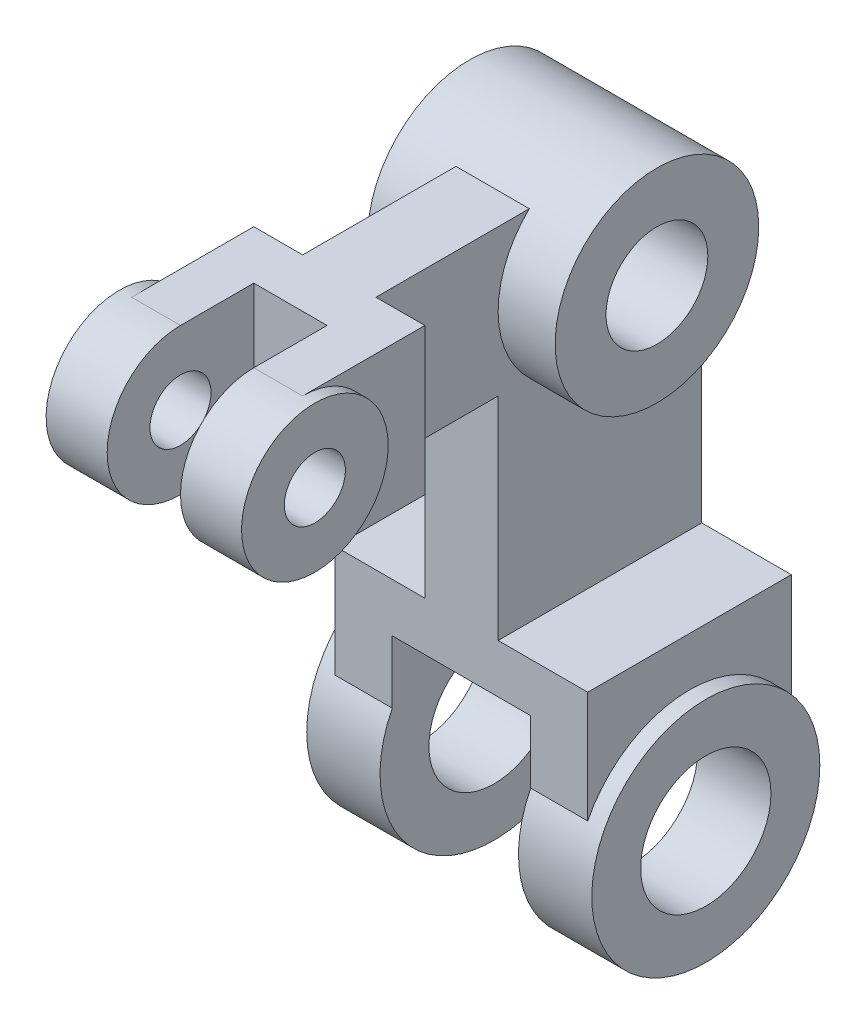
ISO-10303-21;
HEADER;
FILE_DESCRIPTION(('STEP AP214'),'2;1');
FILE_NAME('part.step','',(''),(''),'','','');
FILE_SCHEMA(('AUTOMOTIVE_DESIGN { 1 0 10303 214 1 1 1 1 }'));
ENDSEC;
DATA;
#1=APPLICATION_CONTEXT('core data for automotive mechanical design processes');
#2=APPLICATION_PROTOCOL_DEFINITION('international standard','automotive_design',2000,#1);
#3=PRODUCT_CONTEXT('',#1,'mechanical');
#4=PRODUCT('Part','Part','',(#3));
#5=PRODUCT_RELATED_PRODUCT_CATEGORY('part','',(#4));
#6=PRODUCT_DEFINITION_FORMATION('','',#4);
#7=PRODUCT_DEFINITION_CONTEXT('part definition',#1,'design');
#8=PRODUCT_DEFINITION('design','',#6,#7);
#9=PRODUCT_DEFINITION_SHAPE('','',#8);
#10=(LENGTH_UNIT() NAMED_UNIT(*) SI_UNIT(.MILLI.,.METRE.));
#11=(NAMED_UNIT(*) PLANE_ANGLE_UNIT() SI_UNIT($,.RADIAN.));
#12=(NAMED_UNIT(*) SI_UNIT($,.STERADIAN.) SOLID_ANGLE_UNIT());
#13=UNCERTAINTY_MEASURE_WITH_UNIT(LENGTH_MEASURE(1.E-05),#10,'distance_accuracy_value','');
#14=(GEOMETRIC_REPRESENTATION_CONTEXT(3) GLOBAL_UNCERTAINTY_ASSIGNED_CONTEXT((#13)) GLOBAL_UNIT_ASSIGNED_CONTEXT((#10,
#11,#12)) REPRESENTATION_CONTEXT('',''));
#15=CARTESIAN_POINT('',(0.,0.,0.));
#16=DIRECTION('',(0.,0.,1.));
#17=DIRECTION('',(1.,0.,0.));
#18=AXIS2_PLACEMENT_3D('',#15,#16,#17);
#19=CARTESIAN_POINT('',(0.,0.,25.));
#20=DIRECTION('',(0.,0.,-1.));
#21=DIRECTION('',(-1.,0.,0.));
#22=AXIS2_PLACEMENT_3D('',#19,#20,#21);
#23=PLANE('',#22);
#24=DIRECTION('',(1.,0.,0.));
#25=VECTOR('',#24,1.);
#26=CARTESIAN_POINT('',(0.,92.,25.));
#27=LINE('',#26,#25);
#28=CARTESIAN_POINT('',(-9.,92.,25.));
#29=VERTEX_POINT('',#28);
#30=CARTESIAN_POINT('',(9.,92.,25.));
#31=VERTEX_POINT('',#30);
#32=EDGE_CURVE('E297',#29,#31,#27,.T.);
#33=ORIENTED_EDGE('',*,*,#32,.F.);
#34=DIRECTION('',(0.,-1.,0.));
#35=VECTOR('',#34,1.);
#36=CARTESIAN_POINT('',(-9.,110.,25.));
#37=LINE('',#36,#35);
#38=CARTESIAN_POINT('',(-8.99999999999999,40.,25.));
#39=VERTEX_POINT('',#38);
#40=EDGE_CURVE('E335',#29,#39,#37,.T.);
#41=ORIENTED_EDGE('',*,*,#40,.T.);
#42=DIRECTION('',(-1.,0.,0.));
#43=VECTOR('',#42,1.);
#44=CARTESIAN_POINT('',(-8.99999999999999,40.,25.));
#45=LINE('',#44,#43);
#46=CARTESIAN_POINT('',(-31.,40.,25.));
#47=VERTEX_POINT('',#46);
#48=EDGE_CURVE('E331',#39,#47,#45,.T.);
#49=ORIENTED_EDGE('',*,*,#48,.T.);
#50=DIRECTION('',(0.,-1.,0.));
#51=VECTOR('',#50,1.);
#52=CARTESIAN_POINT('',(-31.,40.,25.));
#53=LINE('',#52,#51);
#54=CARTESIAN_POINT('',(-31.,12.6095202129185,25.));
#55=VERTEX_POINT('',#54);
#56=EDGE_CURVE('E339',#47,#55,#53,.T.);
#57=ORIENTED_EDGE('',*,*,#56,.T.);
#58=DIRECTION('',(1.,0.,0.));
#59=VECTOR('',#58,1.);
#60=CARTESIAN_POINT('',(-35.,12.6095202129185,25.));
#61=LINE('',#60,#59);
#62=CARTESIAN_POINT('',(-17.,12.6095202129185,25.));
#63=VERTEX_POINT('',#62);
#64=EDGE_CURVE('E314',#55,#63,#61,.T.);
#65=ORIENTED_EDGE('',*,*,#64,.T.);
#66=DIRECTION('',(0.,1.,0.));
#67=VECTOR('',#66,1.);
#68=CARTESIAN_POINT('',(-17.,0.,25.));
#69=LINE('',#68,#67);
#70=CARTESIAN_POINT('',(-17.,28.,25.));
#71=VERTEX_POINT('',#70);
#72=EDGE_CURVE('E336',#63,#71,#69,.T.);
#73=ORIENTED_EDGE('',*,*,#72,.T.);
#74=DIRECTION('',(1.,0.,0.));
#75=VECTOR('',#74,1.);
#76=CARTESIAN_POINT('',(-17.,28.,25.));
#77=LINE('',#76,#75);
#78=CARTESIAN_POINT('',(17.,28.,25.));
#79=VERTEX_POINT('',#78);
#80=EDGE_CURVE('E343',#71,#79,#77,.T.);
#81=ORIENTED_EDGE('',*,*,#80,.T.);
#82=DIRECTION('',(0.,-1.,0.));
#83=VECTOR('',#82,1.);
#84=CARTESIAN_POINT('',(17.,0.,25.));
#85=LINE('',#84,#83);
#86=CARTESIAN_POINT('',(17.,12.6095202129185,25.));
#87=VERTEX_POINT('',#86);
#88=EDGE_CURVE('E341',#79,#87,#85,.T.);
#89=ORIENTED_EDGE('',*,*,#88,.T.);
#90=DIRECTION('',(-1.,0.,0.));
#91=VECTOR('',#90,1.);
#92=CARTESIAN_POINT('',(35.,12.6095202129185,25.));
#93=LINE('',#92,#91);
#94=CARTESIAN_POINT('',(31.,12.6095202129185,25.));
#95=VERTEX_POINT('',#94);
#96=EDGE_CURVE('E328',#95,#87,#93,.T.);
#97=ORIENTED_EDGE('',*,*,#96,.F.);
#98=DIRECTION('',(0.,1.,0.));
#99=VECTOR('',#98,1.);
#100=CARTESIAN_POINT('',(31.,40.,25.));
#101=LINE('',#100,#99);
#102=CARTESIAN_POINT('',(31.,40.,25.));
#103=VERTEX_POINT('',#102);
#104=EDGE_CURVE('E347',#95,#103,#101,.T.);
#105=ORIENTED_EDGE('',*,*,#104,.T.);
#106=DIRECTION('',(-1.,0.,0.));
#107=VECTOR('',#106,1.);
#108=CARTESIAN_POINT('',(8.99999999999999,40.,25.));
#109=LINE('',#108,#107);
#110=CARTESIAN_POINT('',(8.99999999999999,40.,25.));
#111=VERTEX_POINT('',#110);
#112=EDGE_CURVE('E346',#103,#111,#109,.T.);
#113=ORIENTED_EDGE('',*,*,#112,.T.);
#114=DIRECTION('',(0.,1.,0.));
#115=VECTOR('',#114,1.);
#116=CARTESIAN_POINT('',(9.,110.,25.));
#117=LINE('',#116,#115);
#118=EDGE_CURVE('E348',#111,#31,#117,.T.);
#119=ORIENTED_EDGE('',*,*,#118,.T.);
#120=EDGE_LOOP('',(#33,#41,#49,#57,#65,#73,#81,#89,#97,#105,#113,#119));
#121=FACE_BOUND('',#120,.T.);
#122=ADVANCED_FACE('F60',(#121),#23,.F.);
#123=CARTESIAN_POINT('',(23.,110.,0.));
#124=DIRECTION('',(-1.,0.,0.));
#125=DIRECTION('',(0.,0.,1.));
#126=AXIS2_PLACEMENT_3D('',#123,#124,#125);
#127=CYLINDRICAL_SURFACE('',#126,25.);
#128=CARTESIAN_POINT('',(23.,110.,0.));
#129=DIRECTION('',(1.,0.,0.));
#130=DIRECTION('',(0.,0.,-1.));
#131=AXIS2_PLACEMENT_3D('',#128,#129,#130);
#132=CIRCLE('',#131,25.);
#133=CARTESIAN_POINT('',(23.,110.,-25.));
#134=VERTEX_POINT('',#133);
#135=EDGE_CURVE('E402',#134,#134,#132,.T.);
#136=ORIENTED_EDGE('',*,*,#135,.F.);
#137=EDGE_LOOP('',(#136));
#138=FACE_BOUND('',#137,.T.);
#139=CARTESIAN_POINT('',(-23.,110.,0.));
#140=DIRECTION('',(1.,0.,0.));
#141=DIRECTION('',(0.,0.,-1.));
#142=AXIS2_PLACEMENT_3D('',#139,#140,#141);
#143=CIRCLE('',#142,25.);
#144=CARTESIAN_POINT('',(-23.,110.,-25.));
#145=VERTEX_POINT('',#144);
#146=EDGE_CURVE('E396',#145,#145,#143,.T.);
#147=ORIENTED_EDGE('',*,*,#146,.T.);
#148=EDGE_LOOP('',(#147));
#149=FACE_BOUND('',#148,.T.);
#150=DIRECTION('',(-1.,0.,0.));
#151=VECTOR('',#150,1.);
#152=CARTESIAN_POINT('',(23.,128.,17.3493515728975));
#153=LINE('',#152,#151);
#154=CARTESIAN_POINT('',(-9.,128.,17.3493515728975));
#155=VERTEX_POINT('',#154);
#156=CARTESIAN_POINT('',(9.,128.,17.3493515728975));
#157=VERTEX_POINT('',#156);
#158=EDGE_CURVE('E63',#155,#157,#153,.F.);
#159=ORIENTED_EDGE('',*,*,#158,.T.);
#160=CARTESIAN_POINT('',(9.,110.,0.));
#161=DIRECTION('',(-1.,0.,0.));
#162=DIRECTION('',(0.,-1.,0.));
#163=AXIS2_PLACEMENT_3D('',#160,#161,#162);
#164=CIRCLE('',#163,25.);
#165=CARTESIAN_POINT('',(9.,110.,-25.));
#166=VERTEX_POINT('',#165);
#167=EDGE_CURVE('E75',#166,#157,#164,.T.);
#168=ORIENTED_EDGE('',*,*,#167,.F.);
#169=DIRECTION('',(-1.,0.,0.));
#170=VECTOR('',#169,1.);
#171=CARTESIAN_POINT('',(-9.,110.,-25.));
#172=LINE('',#171,#170);
#173=CARTESIAN_POINT('',(-9.,110.,-25.));
#174=VERTEX_POINT('',#173);
#175=EDGE_CURVE('E332',#166,#174,#172,.T.);
#176=ORIENTED_EDGE('',*,*,#175,.T.);
#177=CARTESIAN_POINT('',(-9.,110.,0.));
#178=DIRECTION('',(1.,0.,0.));
#179=DIRECTION('',(0.,1.,0.));
#180=AXIS2_PLACEMENT_3D('',#177,#178,#179);
#181=CIRCLE('',#180,25.);
#182=EDGE_CURVE('E394',#155,#174,#181,.T.);
#183=ORIENTED_EDGE('',*,*,#182,.F.);
#184=EDGE_LOOP('',(#159,#168,#176,#183));
#185=FACE_BOUND('',#184,.T.);
#186=ADVANCED_FACE('F56',(#138,#149,#185),#127,.T.);
#187=CARTESIAN_POINT('',(23.,110.,0.));
#188=DIRECTION('',(-1.,0.,0.));
#189=DIRECTION('',(0.,0.,1.));
#190=AXIS2_PLACEMENT_3D('',#187,#188,#189);
#191=CYLINDRICAL_SURFACE('',#190,12.5);
#192=CARTESIAN_POINT('',(23.,110.,0.));
#193=DIRECTION('',(1.,0.,0.));
#194=DIRECTION('',(0.,0.,-1.));
#195=AXIS2_PLACEMENT_3D('',#192,#193,#194);
#196=CIRCLE('',#195,12.5);
#197=CARTESIAN_POINT('',(23.,110.,-12.5));
#198=VERTEX_POINT('',#197);
#199=EDGE_CURVE('E393',#198,#198,#196,.T.);
#200=ORIENTED_EDGE('',*,*,#199,.T.);
#201=EDGE_LOOP('',(#200));
#202=FACE_BOUND('',#201,.T.);
#203=CARTESIAN_POINT('',(-23.,110.,0.));
#204=DIRECTION('',(1.,0.,0.));
#205=DIRECTION('',(0.,0.,-1.));
#206=AXIS2_PLACEMENT_3D('',#203,#204,#205);
#207=CIRCLE('',#206,12.5);
#208=CARTESIAN_POINT('',(-23.,110.,-12.5));
#209=VERTEX_POINT('',#208);
#210=EDGE_CURVE('E391',#209,#209,#207,.T.);
#211=ORIENTED_EDGE('',*,*,#210,.F.);
#212=EDGE_LOOP('',(#211));
#213=FACE_BOUND('',#212,.T.);
#214=ADVANCED_FACE('F480',(#202,#213),#191,.F.);
#215=CARTESIAN_POINT('',(0.,0.,-25.));
#216=DIRECTION('',(0.,0.,-1.));
#217=DIRECTION('',(-1.,0.,0.));
#218=AXIS2_PLACEMENT_3D('',#215,#216,#217);
#219=PLANE('',#218);
#220=DIRECTION('',(1.,0.,0.));
#221=VECTOR('',#220,1.);
#222=CARTESIAN_POINT('',(-35.,12.6095202129185,-25.));
#223=LINE('',#222,#221);
#224=CARTESIAN_POINT('',(-31.,12.6095202129185,-25.));
#225=VERTEX_POINT('',#224);
#226=CARTESIAN_POINT('',(-17.,12.6095202129185,-25.));
#227=VERTEX_POINT('',#226);
#228=EDGE_CURVE('E313',#225,#227,#223,.T.);
#229=ORIENTED_EDGE('',*,*,#228,.F.);
#230=DIRECTION('',(0.,-1.,0.));
#231=VECTOR('',#230,1.);
#232=CARTESIAN_POINT('',(-31.,40.,-25.));
#233=LINE('',#232,#231);
#234=CARTESIAN_POINT('',(-31.,40.,-25.));
#235=VERTEX_POINT('',#234);
#236=EDGE_CURVE('E359',#235,#225,#233,.T.);
#237=ORIENTED_EDGE('',*,*,#236,.F.);
#238=DIRECTION('',(-1.,0.,0.));
#239=VECTOR('',#238,1.);
#240=CARTESIAN_POINT('',(-8.99999999999999,40.,-25.));
#241=LINE('',#240,#239);
#242=CARTESIAN_POINT('',(-8.99999999999999,40.,-25.));
#243=VERTEX_POINT('',#242);
#244=EDGE_CURVE('E356',#243,#235,#241,.T.);
#245=ORIENTED_EDGE('',*,*,#244,.F.);
#246=DIRECTION('',(0.,-1.,0.));
#247=VECTOR('',#246,1.);
#248=CARTESIAN_POINT('',(-9.,110.,-25.));
#249=LINE('',#248,#247);
#250=EDGE_CURVE('E358',#174,#243,#249,.T.);
#251=ORIENTED_EDGE('',*,*,#250,.F.);
#252=ORIENTED_EDGE('',*,*,#175,.F.);
#253=DIRECTION('',(0.,1.,0.));
#254=VECTOR('',#253,1.);
#255=CARTESIAN_POINT('',(9.,110.,-25.));
#256=LINE('',#255,#254);
#257=CARTESIAN_POINT('',(8.99999999999999,40.,-25.));
#258=VERTEX_POINT('',#257);
#259=EDGE_CURVE('E333',#258,#166,#256,.T.);
#260=ORIENTED_EDGE('',*,*,#259,.F.);
#261=DIRECTION('',(-1.,0.,0.));
#262=VECTOR('',#261,1.);
#263=CARTESIAN_POINT('',(8.99999999999999,40.,-25.));
#264=LINE('',#263,#262);
#265=CARTESIAN_POINT('',(31.,40.,-25.));
#266=VERTEX_POINT('',#265);
#267=EDGE_CURVE('E373',#266,#258,#264,.T.);
#268=ORIENTED_EDGE('',*,*,#267,.F.);
#269=DIRECTION('',(0.,1.,0.));
#270=VECTOR('',#269,1.);
#271=CARTESIAN_POINT('',(31.,40.,-25.));
#272=LINE('',#271,#270);
#273=CARTESIAN_POINT('',(31.,12.6095202129185,-25.));
#274=VERTEX_POINT('',#273);
#275=EDGE_CURVE('E371',#274,#266,#272,.T.);
#276=ORIENTED_EDGE('',*,*,#275,.F.);
#277=DIRECTION('',(-1.,0.,0.));
#278=VECTOR('',#277,1.);
#279=CARTESIAN_POINT('',(35.,12.6095202129185,-25.));
#280=LINE('',#279,#278);
#281=CARTESIAN_POINT('',(17.,12.6095202129185,-25.));
#282=VERTEX_POINT('',#281);
#283=EDGE_CURVE('E404',#274,#282,#280,.T.);
#284=ORIENTED_EDGE('',*,*,#283,.T.);
#285=DIRECTION('',(0.,-1.,0.));
#286=VECTOR('',#285,1.);
#287=CARTESIAN_POINT('',(17.,0.,-25.));
#288=LINE('',#287,#286);
#289=CARTESIAN_POINT('',(17.,28.,-25.));
#290=VERTEX_POINT('',#289);
#291=EDGE_CURVE('E366',#290,#282,#288,.T.);
#292=ORIENTED_EDGE('',*,*,#291,.F.);
#293=DIRECTION('',(1.,0.,0.));
#294=VECTOR('',#293,1.);
#295=CARTESIAN_POINT('',(-17.,28.,-25.));
#296=LINE('',#295,#294);
#297=CARTESIAN_POINT('',(-17.,28.,-25.));
#298=VERTEX_POINT('',#297);
#299=EDGE_CURVE('E364',#298,#290,#296,.T.);
#300=ORIENTED_EDGE('',*,*,#299,.F.);
#301=DIRECTION('',(0.,1.,0.));
#302=VECTOR('',#301,1.);
#303=CARTESIAN_POINT('',(-17.,0.,-25.));
#304=LINE('',#303,#302);
#305=EDGE_CURVE('E362',#227,#298,#304,.T.);
#306=ORIENTED_EDGE('',*,*,#305,.F.);
#307=EDGE_LOOP('',(#229,#237,#245,#251,#252,#260,#268,#276,#284,#292,#300,#306));
#308=FACE_BOUND('',#307,.T.);
#309=ADVANCED_FACE('F485',(#308),#219,.T.);
#310=CARTESIAN_POINT('',(23.,110.,0.));
#311=DIRECTION('',(1.,0.,0.));
#312=DIRECTION('',(0.,0.,-1.));
#313=AXIS2_PLACEMENT_3D('',#310,#311,#312);
#314=PLANE('',#313);
#315=ORIENTED_EDGE('',*,*,#135,.T.);
#316=EDGE_LOOP('',(#315));
#317=FACE_BOUND('',#316,.T.);
#318=ORIENTED_EDGE('',*,*,#199,.F.);
#319=EDGE_LOOP('',(#318));
#320=FACE_BOUND('',#319,.T.);
#321=ADVANCED_FACE('F482',(#317,#320),#314,.T.);
#322=CARTESIAN_POINT('',(-23.,110.,0.));
#323=DIRECTION('',(1.,0.,0.));
#324=DIRECTION('',(0.,0.,-1.));
#325=AXIS2_PLACEMENT_3D('',#322,#323,#324);
#326=PLANE('',#325);
#327=ORIENTED_EDGE('',*,*,#146,.F.);
#328=EDGE_LOOP('',(#327));
#329=FACE_BOUND('',#328,.T.);
#330=ORIENTED_EDGE('',*,*,#210,.T.);
#331=EDGE_LOOP('',(#330));
#332=FACE_BOUND('',#331,.T.);
#333=ADVANCED_FACE('F491',(#329,#332),#326,.F.);
#334=CARTESIAN_POINT('',(-9.,110.,25.));
#335=DIRECTION('',(1.,0.,0.));
#336=DIRECTION('',(0.,1.,0.));
#337=AXIS2_PLACEMENT_3D('',#334,#335,#336);
#338=PLANE('',#337);
#339=ORIENTED_EDGE('',*,*,#182,.T.);
#340=ORIENTED_EDGE('',*,*,#250,.T.);
#341=DIRECTION('',(0.,0.,-1.));
#342=VECTOR('',#341,1.);
#343=CARTESIAN_POINT('',(-8.99999999999999,40.,25.));
#344=LINE('',#343,#342);
#345=EDGE_CURVE('E389',#39,#243,#344,.T.);
#346=ORIENTED_EDGE('',*,*,#345,.F.);
#347=ORIENTED_EDGE('',*,*,#40,.F.);
#348=DIRECTION('',(0.,0.,1.));
#349=VECTOR('',#348,1.);
#350=CARTESIAN_POINT('',(-9.,92.,0.));
#351=LINE('',#350,#349);
#352=CARTESIAN_POINT('',(-8.99999999999999,92.,55.));
#353=VERTEX_POINT('',#352);
#354=EDGE_CURVE('E277',#29,#353,#351,.T.);
#355=ORIENTED_EDGE('',*,*,#354,.T.);
#356=DIRECTION('',(0.,-1.,0.));
#357=VECTOR('',#356,1.);
#358=CARTESIAN_POINT('',(-8.99999999999999,128.,55.));
#359=LINE('',#358,#357);
#360=CARTESIAN_POINT('',(-8.99999999999999,128.,55.));
#361=VERTEX_POINT('',#360);
#362=EDGE_CURVE('E285',#361,#353,#359,.T.);
#363=ORIENTED_EDGE('',*,*,#362,.F.);
#364=DIRECTION('',(0.,0.,1.));
#365=VECTOR('',#364,1.);
#366=CARTESIAN_POINT('',(-9.,128.,0.));
#367=LINE('',#366,#365);
#368=EDGE_CURVE('E247',#155,#361,#367,.T.);
#369=ORIENTED_EDGE('',*,*,#368,.F.);
#370=EDGE_LOOP('',(#339,#340,#346,#347,#355,#363,#369));
#371=FACE_BOUND('',#370,.T.);
#372=ADVANCED_FACE('F411',(#371),#338,.F.);
#373=CARTESIAN_POINT('',(-8.99999999999999,40.,25.));
#374=DIRECTION('',(0.,-1.,0.));
#375=DIRECTION('',(1.,0.,0.));
#376=AXIS2_PLACEMENT_3D('',#373,#374,#375);
#377=PLANE('',#376);
#378=ORIENTED_EDGE('',*,*,#244,.T.);
#379=DIRECTION('',(0.,0.,-1.));
#380=VECTOR('',#379,1.);
#381=CARTESIAN_POINT('',(-31.,40.,25.));
#382=LINE('',#381,#380);
#383=EDGE_CURVE('E384',#47,#235,#382,.T.);
#384=ORIENTED_EDGE('',*,*,#383,.F.);
#385=ORIENTED_EDGE('',*,*,#48,.F.);
#386=ORIENTED_EDGE('',*,*,#345,.T.);
#387=EDGE_LOOP('',(#378,#384,#385,#386));
#388=FACE_BOUND('',#387,.T.);
#389=ADVANCED_FACE('F636',(#388),#377,.F.);
#390=CARTESIAN_POINT('',(-31.,40.,25.));
#391=DIRECTION('',(1.,0.,0.));
#392=DIRECTION('',(0.,1.,0.));
#393=AXIS2_PLACEMENT_3D('',#390,#391,#392);
#394=PLANE('',#393);
#395=ORIENTED_EDGE('',*,*,#236,.T.);
#396=CARTESIAN_POINT('',(-31.,0.,0.));
#397=DIRECTION('',(1.,0.,0.));
#398=DIRECTION('',(0.,1.,0.));
#399=AXIS2_PLACEMENT_3D('',#396,#397,#398);
#400=CIRCLE('',#399,28.);
#401=EDGE_CURVE('E78',#225,#55,#400,.T.);
#402=ORIENTED_EDGE('',*,*,#401,.T.);
#403=ORIENTED_EDGE('',*,*,#56,.F.);
#404=ORIENTED_EDGE('',*,*,#383,.T.);
#405=EDGE_LOOP('',(#395,#402,#403,#404));
#406=FACE_BOUND('',#405,.T.);
#407=ADVANCED_FACE('F504',(#406),#394,.F.);
#408=CARTESIAN_POINT('',(-17.,0.,25.));
#409=DIRECTION('',(-1.,0.,0.));
#410=DIRECTION('',(0.,0.,1.));
#411=AXIS2_PLACEMENT_3D('',#408,#409,#410);
#412=PLANE('',#411);
#413=CARTESIAN_POINT('',(-17.,0.,0.));
#414=DIRECTION('',(1.,0.,0.));
#415=DIRECTION('',(0.,0.,-1.));
#416=AXIS2_PLACEMENT_3D('',#413,#414,#415);
#417=CIRCLE('',#416,16.);
#418=CARTESIAN_POINT('',(-17.,0.,-16.));
#419=VERTEX_POINT('',#418);
#420=EDGE_CURVE('E300',#419,#419,#417,.T.);
#421=ORIENTED_EDGE('',*,*,#420,.F.);
#422=EDGE_LOOP('',(#421));
#423=FACE_BOUND('',#422,.T.);
#424=ORIENTED_EDGE('',*,*,#72,.F.);
#425=CARTESIAN_POINT('',(-17.,0.,0.));
#426=DIRECTION('',(1.,0.,0.));
#427=DIRECTION('',(0.,0.,-1.));
#428=AXIS2_PLACEMENT_3D('',#425,#426,#427);
#429=CIRCLE('',#428,28.);
#430=EDGE_CURVE('E305',#63,#227,#429,.T.);
#431=ORIENTED_EDGE('',*,*,#430,.T.);
#432=ORIENTED_EDGE('',*,*,#305,.T.);
#433=DIRECTION('',(0.,0.,-1.));
#434=VECTOR('',#433,1.);
#435=CARTESIAN_POINT('',(-17.,28.,25.));
#436=LINE('',#435,#434);
#437=EDGE_CURVE('E382',#71,#298,#436,.T.);
#438=ORIENTED_EDGE('',*,*,#437,.F.);
#439=EDGE_LOOP('',(#424,#431,#432,#438));
#440=FACE_BOUND('',#439,.T.);
#441=ADVANCED_FACE('F507',(#423,#440),#412,.F.);
#442=CARTESIAN_POINT('',(-17.,28.,25.));
#443=DIRECTION('',(0.,1.,0.));
#444=DIRECTION('',(0.,0.,1.));
#445=AXIS2_PLACEMENT_3D('',#442,#443,#444);
#446=PLANE('',#445);
#447=ORIENTED_EDGE('',*,*,#299,.T.);
#448=DIRECTION('',(0.,0.,-1.));
#449=VECTOR('',#448,1.);
#450=CARTESIAN_POINT('',(17.,28.,25.));
#451=LINE('',#450,#449);
#452=EDGE_CURVE('E381',#79,#290,#451,.T.);
#453=ORIENTED_EDGE('',*,*,#452,.F.);
#454=ORIENTED_EDGE('',*,*,#80,.F.);
#455=ORIENTED_EDGE('',*,*,#437,.T.);
#456=EDGE_LOOP('',(#447,#453,#454,#455));
#457=FACE_BOUND('',#456,.T.);
#458=ADVANCED_FACE('F511',(#457),#446,.F.);
#459=CARTESIAN_POINT('',(17.,0.,25.));
#460=DIRECTION('',(1.,0.,0.));
#461=DIRECTION('',(0.,0.,-1.));
#462=AXIS2_PLACEMENT_3D('',#459,#460,#461);
#463=PLANE('',#462);
#464=CARTESIAN_POINT('',(17.,0.,0.));
#465=DIRECTION('',(1.,0.,0.));
#466=DIRECTION('',(0.,0.,-1.));
#467=AXIS2_PLACEMENT_3D('',#464,#465,#466);
#468=CIRCLE('',#467,16.);
#469=CARTESIAN_POINT('',(17.,0.,-16.));
#470=VERTEX_POINT('',#469);
#471=EDGE_CURVE('E316',#470,#470,#468,.T.);
#472=ORIENTED_EDGE('',*,*,#471,.T.);
#473=EDGE_LOOP('',(#472));
#474=FACE_BOUND('',#473,.T.);
#475=ORIENTED_EDGE('',*,*,#452,.T.);
#476=ORIENTED_EDGE('',*,*,#291,.T.);
#477=CARTESIAN_POINT('',(17.,0.,0.));
#478=DIRECTION('',(1.,0.,0.));
#479=DIRECTION('',(0.,0.,-1.));
#480=AXIS2_PLACEMENT_3D('',#477,#478,#479);
#481=CIRCLE('',#480,28.);
#482=EDGE_CURVE('E319',#87,#282,#481,.T.);
#483=ORIENTED_EDGE('',*,*,#482,.F.);
#484=ORIENTED_EDGE('',*,*,#88,.F.);
#485=EDGE_LOOP('',(#475,#476,#483,#484));
#486=FACE_BOUND('',#485,.T.);
#487=ADVANCED_FACE('F516',(#474,#486),#463,.F.);
#488=CARTESIAN_POINT('',(31.,40.,25.));
#489=DIRECTION('',(-1.,0.,0.));
#490=DIRECTION('',(0.,-1.,0.));
#491=AXIS2_PLACEMENT_3D('',#488,#489,#490);
#492=PLANE('',#491);
#493=CARTESIAN_POINT('',(31.,0.,0.));
#494=DIRECTION('',(-1.,0.,0.));
#495=DIRECTION('',(0.,-1.,0.));
#496=AXIS2_PLACEMENT_3D('',#493,#494,#495);
#497=CIRCLE('',#496,28.);
#498=EDGE_CURVE('E326',#274,#95,#497,.F.);
#499=ORIENTED_EDGE('',*,*,#498,.F.);
#500=ORIENTED_EDGE('',*,*,#275,.T.);
#501=DIRECTION('',(0.,0.,-1.));
#502=VECTOR('',#501,1.);
#503=CARTESIAN_POINT('',(31.,40.,25.));
#504=LINE('',#503,#502);
#505=EDGE_CURVE('E378',#103,#266,#504,.T.);
#506=ORIENTED_EDGE('',*,*,#505,.F.);
#507=ORIENTED_EDGE('',*,*,#104,.F.);
#508=EDGE_LOOP('',(#499,#500,#506,#507));
#509=FACE_BOUND('',#508,.T.);
#510=ADVANCED_FACE('F468',(#509),#492,.F.);
#511=CARTESIAN_POINT('',(8.99999999999999,40.,25.));
#512=DIRECTION('',(0.,-1.,0.));
#513=DIRECTION('',(1.,0.,0.));
#514=AXIS2_PLACEMENT_3D('',#511,#512,#513);
#515=PLANE('',#514);
#516=ORIENTED_EDGE('',*,*,#267,.T.);
#517=DIRECTION('',(0.,0.,-1.));
#518=VECTOR('',#517,1.);
#519=CARTESIAN_POINT('',(8.99999999999999,40.,25.));
#520=LINE('',#519,#518);
#521=EDGE_CURVE('E355',#111,#258,#520,.T.);
#522=ORIENTED_EDGE('',*,*,#521,.F.);
#523=ORIENTED_EDGE('',*,*,#112,.F.);
#524=ORIENTED_EDGE('',*,*,#505,.T.);
#525=EDGE_LOOP('',(#516,#522,#523,#524));
#526=FACE_BOUND('',#525,.T.);
#527=ADVANCED_FACE('F454',(#526),#515,.F.);
#528=CARTESIAN_POINT('',(9.,110.,25.));
#529=DIRECTION('',(-1.,0.,0.));
#530=DIRECTION('',(0.,-1.,0.));
#531=AXIS2_PLACEMENT_3D('',#528,#529,#530);
#532=PLANE('',#531);
#533=ORIENTED_EDGE('',*,*,#167,.T.);
#534=DIRECTION('',(0.,0.,-1.));
#535=VECTOR('',#534,1.);
#536=CARTESIAN_POINT('',(9.,128.,0.));
#537=LINE('',#536,#535);
#538=CARTESIAN_POINT('',(9.00000000000001,128.,55.));
#539=VERTEX_POINT('',#538);
#540=EDGE_CURVE('E250',#539,#157,#537,.T.);
#541=ORIENTED_EDGE('',*,*,#540,.F.);
#542=DIRECTION('',(0.,-1.,0.));
#543=VECTOR('',#542,1.);
#544=CARTESIAN_POINT('',(9.00000000000001,128.,55.));
#545=LINE('',#544,#543);
#546=CARTESIAN_POINT('',(9.00000000000001,92.,55.));
#547=VERTEX_POINT('',#546);
#548=EDGE_CURVE('E288',#539,#547,#545,.T.);
#549=ORIENTED_EDGE('',*,*,#548,.T.);
#550=DIRECTION('',(0.,0.,-1.));
#551=VECTOR('',#550,1.);
#552=CARTESIAN_POINT('',(9.,92.,0.));
#553=LINE('',#552,#551);
#554=EDGE_CURVE('E272',#547,#31,#553,.T.);
#555=ORIENTED_EDGE('',*,*,#554,.T.);
#556=ORIENTED_EDGE('',*,*,#118,.F.);
#557=ORIENTED_EDGE('',*,*,#521,.T.);
#558=ORIENTED_EDGE('',*,*,#259,.T.);
#559=EDGE_LOOP('',(#533,#541,#549,#555,#556,#557,#558));
#560=FACE_BOUND('',#559,.T.);
#561=ADVANCED_FACE('F455',(#560),#532,.F.);
#562=CARTESIAN_POINT('',(35.,0.,0.));
#563=DIRECTION('',(-1.,0.,0.));
#564=DIRECTION('',(0.,0.,1.));
#565=AXIS2_PLACEMENT_3D('',#562,#563,#564);
#566=CYLINDRICAL_SURFACE('',#565,16.);
#567=CARTESIAN_POINT('',(35.,0.,0.));
#568=DIRECTION('',(1.,0.,0.));
#569=DIRECTION('',(0.,0.,-1.));
#570=AXIS2_PLACEMENT_3D('',#567,#568,#569);
#571=CIRCLE('',#570,16.);
#572=CARTESIAN_POINT('',(35.,0.,-16.));
#573=VERTEX_POINT('',#572);
#574=EDGE_CURVE('E320',#573,#573,#571,.T.);
#575=ORIENTED_EDGE('',*,*,#574,.T.);
#576=EDGE_LOOP('',(#575));
#577=FACE_BOUND('',#576,.T.);
#578=ORIENTED_EDGE('',*,*,#471,.F.);
#579=EDGE_LOOP('',(#578));
#580=FACE_BOUND('',#579,.T.);
#581=ADVANCED_FACE('F452',(#577,#580),#566,.F.);
#582=CARTESIAN_POINT('',(35.,0.,0.));
#583=DIRECTION('',(-1.,0.,0.));
#584=DIRECTION('',(0.,0.,1.));
#585=AXIS2_PLACEMENT_3D('',#582,#583,#584);
#586=CYLINDRICAL_SURFACE('',#585,28.);
#587=CARTESIAN_POINT('',(35.,0.,0.));
#588=DIRECTION('',(1.,0.,0.));
#589=DIRECTION('',(0.,0.,-1.));
#590=AXIS2_PLACEMENT_3D('',#587,#588,#589);
#591=CIRCLE('',#590,28.);
#592=CARTESIAN_POINT('',(35.,0.,-28.));
#593=VERTEX_POINT('',#592);
#594=EDGE_CURVE('E323',#593,#593,#591,.T.);
#595=ORIENTED_EDGE('',*,*,#594,.F.);
#596=EDGE_LOOP('',(#595));
#597=FACE_BOUND('',#596,.T.);
#598=ORIENTED_EDGE('',*,*,#498,.T.);
#599=ORIENTED_EDGE('',*,*,#96,.T.);
#600=ORIENTED_EDGE('',*,*,#482,.T.);
#601=ORIENTED_EDGE('',*,*,#283,.F.);
#602=EDGE_LOOP('',(#598,#599,#600,#601));
#603=FACE_BOUND('',#602,.T.);
#604=ADVANCED_FACE('F464',(#597,#603),#586,.T.);
#605=CARTESIAN_POINT('',(35.,0.,0.));
#606=DIRECTION('',(1.,0.,0.));
#607=DIRECTION('',(0.,0.,-1.));
#608=AXIS2_PLACEMENT_3D('',#605,#606,#607);
#609=PLANE('',#608);
#610=ORIENTED_EDGE('',*,*,#594,.T.);
#611=EDGE_LOOP('',(#610));
#612=FACE_BOUND('',#611,.T.);
#613=ORIENTED_EDGE('',*,*,#574,.F.);
#614=EDGE_LOOP('',(#613));
#615=FACE_BOUND('',#614,.T.);
#616=ADVANCED_FACE('F608',(#612,#615),#609,.T.);
#617=CARTESIAN_POINT('',(-35.,0.,0.));
#618=DIRECTION('',(1.,0.,0.));
#619=DIRECTION('',(0.,0.,-1.));
#620=AXIS2_PLACEMENT_3D('',#617,#618,#619);
#621=CYLINDRICAL_SURFACE('',#620,28.);
#622=CARTESIAN_POINT('',(-35.,0.,0.));
#623=DIRECTION('',(1.,0.,0.));
#624=DIRECTION('',(0.,0.,-1.));
#625=AXIS2_PLACEMENT_3D('',#622,#623,#624);
#626=CIRCLE('',#625,28.);
#627=CARTESIAN_POINT('',(-35.,0.,-28.));
#628=VERTEX_POINT('',#627);
#629=EDGE_CURVE('E304',#628,#628,#626,.T.);
#630=ORIENTED_EDGE('',*,*,#629,.T.);
#631=EDGE_LOOP('',(#630));
#632=FACE_BOUND('',#631,.T.);
#633=ORIENTED_EDGE('',*,*,#64,.F.);
#634=ORIENTED_EDGE('',*,*,#401,.F.);
#635=ORIENTED_EDGE('',*,*,#228,.T.);
#636=ORIENTED_EDGE('',*,*,#430,.F.);
#637=EDGE_LOOP('',(#633,#634,#635,#636));
#638=FACE_BOUND('',#637,.T.);
#639=ADVANCED_FACE('F503',(#632,#638),#621,.T.);
#640=CARTESIAN_POINT('',(-35.,0.,0.));
#641=DIRECTION('',(1.,0.,0.));
#642=DIRECTION('',(0.,0.,-1.));
#643=AXIS2_PLACEMENT_3D('',#640,#641,#642);
#644=CYLINDRICAL_SURFACE('',#643,16.);
#645=CARTESIAN_POINT('',(-35.,0.,0.));
#646=DIRECTION('',(1.,0.,0.));
#647=DIRECTION('',(0.,0.,-1.));
#648=AXIS2_PLACEMENT_3D('',#645,#646,#647);
#649=CIRCLE('',#648,16.);
#650=CARTESIAN_POINT('',(-35.,0.,-16.));
#651=VERTEX_POINT('',#650);
#652=EDGE_CURVE('E296',#651,#651,#649,.T.);
#653=ORIENTED_EDGE('',*,*,#652,.F.);
#654=EDGE_LOOP('',(#653));
#655=FACE_BOUND('',#654,.T.);
#656=ORIENTED_EDGE('',*,*,#420,.T.);
#657=EDGE_LOOP('',(#656));
#658=FACE_BOUND('',#657,.T.);
#659=ADVANCED_FACE('F602',(#655,#658),#644,.F.);
#660=CARTESIAN_POINT('',(-35.,0.,0.));
#661=DIRECTION('',(1.,0.,0.));
#662=DIRECTION('',(0.,0.,-1.));
#663=AXIS2_PLACEMENT_3D('',#660,#661,#662);
#664=PLANE('',#663);
#665=ORIENTED_EDGE('',*,*,#652,.T.);
#666=EDGE_LOOP('',(#665));
#667=FACE_BOUND('',#666,.T.);
#668=ORIENTED_EDGE('',*,*,#629,.F.);
#669=EDGE_LOOP('',(#668));
#670=FACE_BOUND('',#669,.T.);
#671=ADVANCED_FACE('F584',(#667,#670),#664,.F.);
#672=CARTESIAN_POINT('',(0.,128.,0.));
#673=DIRECTION('',(0.,1.,0.));
#674=DIRECTION('',(0.,0.,1.));
#675=AXIS2_PLACEMENT_3D('',#672,#673,#674);
#676=PLANE('',#675);
#677=ORIENTED_EDGE('',*,*,#158,.F.);
#678=ORIENTED_EDGE('',*,*,#368,.T.);
#679=DIRECTION('',(-1.,0.,0.));
#680=VECTOR('',#679,1.);
#681=CARTESIAN_POINT('',(-8.99999999999999,128.,55.));
#682=LINE('',#681,#680);
#683=CARTESIAN_POINT('',(-21.,128.,55.));
#684=VERTEX_POINT('',#683);
#685=EDGE_CURVE('E253',#361,#684,#682,.T.);
#686=ORIENTED_EDGE('',*,*,#685,.T.);
#687=DIRECTION('',(0.,0.,1.));
#688=VECTOR('',#687,1.);
#689=CARTESIAN_POINT('',(-21.,128.,55.));
#690=LINE('',#689,#688);
#691=CARTESIAN_POINT('',(-21.,128.,85.));
#692=VERTEX_POINT('',#691);
#693=EDGE_CURVE('E278',#684,#692,#690,.T.);
#694=ORIENTED_EDGE('',*,*,#693,.T.);
#695=DIRECTION('',(1.,0.,0.));
#696=VECTOR('',#695,1.);
#697=CARTESIAN_POINT('',(-21.,128.,85.));
#698=LINE('',#697,#696);
#699=CARTESIAN_POINT('',(-9.,128.,85.));
#700=VERTEX_POINT('',#699);
#701=EDGE_CURVE('E424',#692,#700,#698,.T.);
#702=ORIENTED_EDGE('',*,*,#701,.T.);
#703=DIRECTION('',(0.,0.,-1.));
#704=VECTOR('',#703,1.);
#705=CARTESIAN_POINT('',(-9.,128.,85.));
#706=LINE('',#705,#704);
#707=CARTESIAN_POINT('',(-9.,128.,67.));
#708=VERTEX_POINT('',#707);
#709=EDGE_CURVE('E238',#700,#708,#706,.T.);
#710=ORIENTED_EDGE('',*,*,#709,.T.);
#711=DIRECTION('',(1.,0.,0.));
#712=VECTOR('',#711,1.);
#713=CARTESIAN_POINT('',(-9.,128.,67.));
#714=LINE('',#713,#712);
#715=CARTESIAN_POINT('',(9.,128.,67.));
#716=VERTEX_POINT('',#715);
#717=EDGE_CURVE('E240',#708,#716,#714,.T.);
#718=ORIENTED_EDGE('',*,*,#717,.T.);
#719=DIRECTION('',(0.,0.,1.));
#720=VECTOR('',#719,1.);
#721=CARTESIAN_POINT('',(9.,128.,67.));
#722=LINE('',#721,#720);
#723=CARTESIAN_POINT('',(9.,128.,85.));
#724=VERTEX_POINT('',#723);
#725=EDGE_CURVE('E224',#716,#724,#722,.T.);
#726=ORIENTED_EDGE('',*,*,#725,.T.);
#727=DIRECTION('',(1.,0.,0.));
#728=VECTOR('',#727,1.);
#729=CARTESIAN_POINT('',(9.,128.,85.));
#730=LINE('',#729,#728);
#731=CARTESIAN_POINT('',(21.,128.,85.));
#732=VERTEX_POINT('',#731);
#733=EDGE_CURVE('E213',#724,#732,#730,.T.);
#734=ORIENTED_EDGE('',*,*,#733,.T.);
#735=DIRECTION('',(0.,0.,-1.));
#736=VECTOR('',#735,1.);
#737=CARTESIAN_POINT('',(21.,128.,55.));
#738=LINE('',#737,#736);
#739=CARTESIAN_POINT('',(21.,128.,55.));
#740=VERTEX_POINT('',#739);
#741=EDGE_CURVE('E225',#732,#740,#738,.T.);
#742=ORIENTED_EDGE('',*,*,#741,.T.);
#743=DIRECTION('',(-1.,0.,0.));
#744=VECTOR('',#743,1.);
#745=CARTESIAN_POINT('',(9.00000000000001,128.,55.));
#746=LINE('',#745,#744);
#747=EDGE_CURVE('E243',#740,#539,#746,.T.);
#748=ORIENTED_EDGE('',*,*,#747,.T.);
#749=ORIENTED_EDGE('',*,*,#540,.T.);
#750=EDGE_LOOP('',(#677,#678,#686,#694,#702,#710,#718,#726,#734,#742,#748,#749));
#751=FACE_BOUND('',#750,.T.);
#752=ADVANCED_FACE('F234',(#751),#676,.T.);
#753=CARTESIAN_POINT('',(0.,92.,0.));
#754=DIRECTION('',(0.,1.,0.));
#755=DIRECTION('',(0.,0.,1.));
#756=AXIS2_PLACEMENT_3D('',#753,#754,#755);
#757=PLANE('',#756);
#758=ORIENTED_EDGE('',*,*,#354,.F.);
#759=ORIENTED_EDGE('',*,*,#32,.T.);
#760=ORIENTED_EDGE('',*,*,#554,.F.);
#761=DIRECTION('',(-1.,0.,0.));
#762=VECTOR('',#761,1.);
#763=CARTESIAN_POINT('',(9.00000000000001,92.,55.));
#764=LINE('',#763,#762);
#765=CARTESIAN_POINT('',(21.,92.,55.));
#766=VERTEX_POINT('',#765);
#767=EDGE_CURVE('E271',#766,#547,#764,.T.);
#768=ORIENTED_EDGE('',*,*,#767,.F.);
#769=DIRECTION('',(0.,0.,-1.));
#770=VECTOR('',#769,1.);
#771=CARTESIAN_POINT('',(21.,92.,55.));
#772=LINE('',#771,#770);
#773=CARTESIAN_POINT('',(21.,92.,85.));
#774=VERTEX_POINT('',#773);
#775=EDGE_CURVE('E267',#774,#766,#772,.T.);
#776=ORIENTED_EDGE('',*,*,#775,.F.);
#777=DIRECTION('',(1.,0.,0.));
#778=VECTOR('',#777,1.);
#779=CARTESIAN_POINT('',(9.,92.,85.));
#780=LINE('',#779,#778);
#781=CARTESIAN_POINT('',(9.,92.,85.));
#782=VERTEX_POINT('',#781);
#783=EDGE_CURVE('E270',#782,#774,#780,.T.);
#784=ORIENTED_EDGE('',*,*,#783,.F.);
#785=DIRECTION('',(0.,0.,1.));
#786=VECTOR('',#785,1.);
#787=CARTESIAN_POINT('',(9.,92.,67.));
#788=LINE('',#787,#786);
#789=CARTESIAN_POINT('',(9.,92.,67.));
#790=VERTEX_POINT('',#789);
#791=EDGE_CURVE('E226',#790,#782,#788,.T.);
#792=ORIENTED_EDGE('',*,*,#791,.F.);
#793=DIRECTION('',(1.,0.,0.));
#794=VECTOR('',#793,1.);
#795=CARTESIAN_POINT('',(-9.,92.,67.));
#796=LINE('',#795,#794);
#797=CARTESIAN_POINT('',(-9.,92.,67.));
#798=VERTEX_POINT('',#797);
#799=EDGE_CURVE('E263',#798,#790,#796,.T.);
#800=ORIENTED_EDGE('',*,*,#799,.F.);
#801=DIRECTION('',(0.,0.,-1.));
#802=VECTOR('',#801,1.);
#803=CARTESIAN_POINT('',(-9.,92.,85.));
#804=LINE('',#803,#802);
#805=CARTESIAN_POINT('',(-9.,92.,85.));
#806=VERTEX_POINT('',#805);
#807=EDGE_CURVE('E257',#806,#798,#804,.T.);
#808=ORIENTED_EDGE('',*,*,#807,.F.);
#809=DIRECTION('',(1.,0.,0.));
#810=VECTOR('',#809,1.);
#811=CARTESIAN_POINT('',(-21.,92.,85.));
#812=LINE('',#811,#810);
#813=CARTESIAN_POINT('',(-21.,92.,85.));
#814=VERTEX_POINT('',#813);
#815=EDGE_CURVE('E260',#814,#806,#812,.T.);
#816=ORIENTED_EDGE('',*,*,#815,.F.);
#817=DIRECTION('',(0.,0.,1.));
#818=VECTOR('',#817,1.);
#819=CARTESIAN_POINT('',(-21.,92.,55.));
#820=LINE('',#819,#818);
#821=CARTESIAN_POINT('',(-21.,92.,55.));
#822=VERTEX_POINT('',#821);
#823=EDGE_CURVE('E255',#822,#814,#820,.T.);
#824=ORIENTED_EDGE('',*,*,#823,.F.);
#825=DIRECTION('',(-1.,0.,0.));
#826=VECTOR('',#825,1.);
#827=CARTESIAN_POINT('',(-8.99999999999999,92.,55.));
#828=LINE('',#827,#826);
#829=EDGE_CURVE('E279',#353,#822,#828,.T.);
#830=ORIENTED_EDGE('',*,*,#829,.F.);
#831=EDGE_LOOP('',(#758,#759,#760,#768,#776,#784,#792,#800,#808,#816,#824,#830));
#832=FACE_BOUND('',#831,.T.);
#833=ADVANCED_FACE('F442',(#832),#757,.F.);
#834=CARTESIAN_POINT('',(-21.,128.,55.));
#835=DIRECTION('',(1.,0.,0.));
#836=DIRECTION('',(0.,0.,-1.));
#837=AXIS2_PLACEMENT_3D('',#834,#835,#836);
#838=PLANE('',#837);
#839=CARTESIAN_POINT('',(-21.,110.,85.));
#840=DIRECTION('',(1.,0.,0.));
#841=DIRECTION('',(0.,0.,-1.));
#842=AXIS2_PLACEMENT_3D('',#839,#840,#841);
#843=CIRCLE('',#842,18.);
#844=EDGE_CURVE('E256',#692,#814,#843,.F.);
#845=ORIENTED_EDGE('',*,*,#844,.F.);
#846=ORIENTED_EDGE('',*,*,#693,.F.);
#847=DIRECTION('',(0.,-1.,0.));
#848=VECTOR('',#847,1.);
#849=CARTESIAN_POINT('',(-21.,128.,55.));
#850=LINE('',#849,#848);
#851=EDGE_CURVE('E251',#684,#822,#850,.T.);
#852=ORIENTED_EDGE('',*,*,#851,.T.);
#853=ORIENTED_EDGE('',*,*,#823,.T.);
#854=EDGE_LOOP('',(#845,#846,#852,#853));
#855=FACE_BOUND('',#854,.T.);
#856=ADVANCED_FACE('F531',(#855),#838,.F.);
#857=CARTESIAN_POINT('',(-9.,128.,85.));
#858=DIRECTION('',(-1.,0.,0.));
#859=DIRECTION('',(0.,0.,1.));
#860=AXIS2_PLACEMENT_3D('',#857,#858,#859);
#861=PLANE('',#860);
#862=CARTESIAN_POINT('',(-9.,110.,85.));
#863=DIRECTION('',(1.,0.,0.));
#864=DIRECTION('',(0.,0.,-1.));
#865=AXIS2_PLACEMENT_3D('',#862,#863,#864);
#866=CIRCLE('',#865,7.5);
#867=CARTESIAN_POINT('',(-9.,110.,77.5));
#868=VERTEX_POINT('',#867);
#869=EDGE_CURVE('E537',#868,#868,#866,.T.);
#870=ORIENTED_EDGE('',*,*,#869,.F.);
#871=EDGE_LOOP('',(#870));
#872=FACE_BOUND('',#871,.T.);
#873=ORIENTED_EDGE('',*,*,#807,.T.);
#874=DIRECTION('',(0.,-1.,0.));
#875=VECTOR('',#874,1.);
#876=CARTESIAN_POINT('',(-9.,128.,67.));
#877=LINE('',#876,#875);
#878=EDGE_CURVE('E294',#708,#798,#877,.T.);
#879=ORIENTED_EDGE('',*,*,#878,.F.);
#880=ORIENTED_EDGE('',*,*,#709,.F.);
#881=CARTESIAN_POINT('',(-9.,110.,85.));
#882=DIRECTION('',(1.,0.,0.));
#883=DIRECTION('',(0.,0.,-1.));
#884=AXIS2_PLACEMENT_3D('',#881,#882,#883);
#885=CIRCLE('',#884,18.);
#886=EDGE_CURVE('E532',#700,#806,#885,.T.);
#887=ORIENTED_EDGE('',*,*,#886,.T.);
#888=EDGE_LOOP('',(#873,#879,#880,#887));
#889=FACE_BOUND('',#888,.T.);
#890=ADVANCED_FACE('F434',(#872,#889),#861,.F.);
#891=CARTESIAN_POINT('',(-9.,128.,67.));
#892=DIRECTION('',(0.,0.,-1.));
#893=DIRECTION('',(-1.,0.,0.));
#894=AXIS2_PLACEMENT_3D('',#891,#892,#893);
#895=PLANE('',#894);
#896=ORIENTED_EDGE('',*,*,#799,.T.);
#897=DIRECTION('',(0.,-1.,0.));
#898=VECTOR('',#897,1.);
#899=CARTESIAN_POINT('',(9.,128.,67.));
#900=LINE('',#899,#898);
#901=EDGE_CURVE('E295',#716,#790,#900,.T.);
#902=ORIENTED_EDGE('',*,*,#901,.F.);
#903=ORIENTED_EDGE('',*,*,#717,.F.);
#904=ORIENTED_EDGE('',*,*,#878,.T.);
#905=EDGE_LOOP('',(#896,#902,#903,#904));
#906=FACE_BOUND('',#905,.T.);
#907=ADVANCED_FACE('F438',(#906),#895,.F.);
#908=CARTESIAN_POINT('',(9.,128.,67.));
#909=DIRECTION('',(1.,0.,0.));
#910=DIRECTION('',(0.,0.,-1.));
#911=AXIS2_PLACEMENT_3D('',#908,#909,#910);
#912=PLANE('',#911);
#913=CARTESIAN_POINT('',(9.,110.,85.));
#914=DIRECTION('',(1.,0.,0.));
#915=DIRECTION('',(0.,0.,-1.));
#916=AXIS2_PLACEMENT_3D('',#913,#914,#915);
#917=CIRCLE('',#916,7.5);
#918=CARTESIAN_POINT('',(9.,110.,77.5));
#919=VERTEX_POINT('',#918);
#920=EDGE_CURVE('E235',#919,#919,#917,.T.);
#921=ORIENTED_EDGE('',*,*,#920,.T.);
#922=EDGE_LOOP('',(#921));
#923=FACE_BOUND('',#922,.T.);
#924=CARTESIAN_POINT('',(9.,110.,85.));
#925=DIRECTION('',(1.,0.,0.));
#926=DIRECTION('',(0.,0.,-1.));
#927=AXIS2_PLACEMENT_3D('',#924,#925,#926);
#928=CIRCLE('',#927,18.);
#929=EDGE_CURVE('E216',#724,#782,#928,.T.);
#930=ORIENTED_EDGE('',*,*,#929,.F.);
#931=ORIENTED_EDGE('',*,*,#725,.F.);
#932=ORIENTED_EDGE('',*,*,#901,.T.);
#933=ORIENTED_EDGE('',*,*,#791,.T.);
#934=EDGE_LOOP('',(#930,#931,#932,#933));
#935=FACE_BOUND('',#934,.T.);
#936=ADVANCED_FACE('F229',(#923,#935),#912,.F.);
#937=CARTESIAN_POINT('',(21.,128.,55.));
#938=DIRECTION('',(-1.,0.,0.));
#939=DIRECTION('',(0.,0.,1.));
#940=AXIS2_PLACEMENT_3D('',#937,#938,#939);
#941=PLANE('',#940);
#942=CARTESIAN_POINT('',(21.,110.,85.));
#943=DIRECTION('',(-1.,0.,0.));
#944=DIRECTION('',(0.,0.,1.));
#945=AXIS2_PLACEMENT_3D('',#942,#943,#944);
#946=CIRCLE('',#945,18.);
#947=EDGE_CURVE('E12',#774,#732,#946,.F.);
#948=ORIENTED_EDGE('',*,*,#947,.F.);
#949=ORIENTED_EDGE('',*,*,#775,.T.);
#950=DIRECTION('',(0.,-1.,0.));
#951=VECTOR('',#950,1.);
#952=CARTESIAN_POINT('',(21.,128.,55.));
#953=LINE('',#952,#951);
#954=EDGE_CURVE('E287',#740,#766,#953,.T.);
#955=ORIENTED_EDGE('',*,*,#954,.F.);
#956=ORIENTED_EDGE('',*,*,#741,.F.);
#957=EDGE_LOOP('',(#948,#949,#955,#956));
#958=FACE_BOUND('',#957,.T.);
#959=ADVANCED_FACE('F443',(#958),#941,.F.);
#960=CARTESIAN_POINT('',(9.00000000000001,128.,55.));
#961=DIRECTION('',(0.,0.,1.));
#962=DIRECTION('',(1.,0.,0.));
#963=AXIS2_PLACEMENT_3D('',#960,#961,#962);
#964=PLANE('',#963);
#965=ORIENTED_EDGE('',*,*,#767,.T.);
#966=ORIENTED_EDGE('',*,*,#548,.F.);
#967=ORIENTED_EDGE('',*,*,#747,.F.);
#968=ORIENTED_EDGE('',*,*,#954,.T.);
#969=EDGE_LOOP('',(#965,#966,#967,#968));
#970=FACE_BOUND('',#969,.T.);
#971=ADVANCED_FACE('F448',(#970),#964,.F.);
#972=CARTESIAN_POINT('',(-8.99999999999999,128.,55.));
#973=DIRECTION('',(0.,0.,1.));
#974=DIRECTION('',(1.,0.,0.));
#975=AXIS2_PLACEMENT_3D('',#972,#973,#974);
#976=PLANE('',#975);
#977=ORIENTED_EDGE('',*,*,#829,.T.);
#978=ORIENTED_EDGE('',*,*,#851,.F.);
#979=ORIENTED_EDGE('',*,*,#685,.F.);
#980=ORIENTED_EDGE('',*,*,#362,.T.);
#981=EDGE_LOOP('',(#977,#978,#979,#980));
#982=FACE_BOUND('',#981,.T.);
#983=ADVANCED_FACE('F419',(#982),#976,.F.);
#984=CARTESIAN_POINT('',(24.,110.,85.));
#985=DIRECTION('',(-1.,0.,0.));
#986=DIRECTION('',(0.,0.,1.));
#987=AXIS2_PLACEMENT_3D('',#984,#985,#986);
#988=CYLINDRICAL_SURFACE('',#987,18.);
#989=CARTESIAN_POINT('',(-24.,110.,85.));
#990=DIRECTION('',(1.,0.,0.));
#991=DIRECTION('',(0.,0.,-1.));
#992=AXIS2_PLACEMENT_3D('',#989,#990,#991);
#993=CIRCLE('',#992,18.);
#994=CARTESIAN_POINT('',(-24.,110.,67.));
#995=VERTEX_POINT('',#994);
#996=EDGE_CURVE('E543',#995,#995,#993,.T.);
#997=ORIENTED_EDGE('',*,*,#996,.T.);
#998=EDGE_LOOP('',(#997));
#999=FACE_BOUND('',#998,.T.);
#1000=ORIENTED_EDGE('',*,*,#844,.T.);
#1001=ORIENTED_EDGE('',*,*,#815,.T.);
#1002=ORIENTED_EDGE('',*,*,#886,.F.);
#1003=ORIENTED_EDGE('',*,*,#701,.F.);
#1004=EDGE_LOOP('',(#1000,#1001,#1002,#1003));
#1005=FACE_BOUND('',#1004,.T.);
#1006=ADVANCED_FACE('F577',(#999,#1005),#988,.T.);
#1007=CARTESIAN_POINT('',(24.,110.,85.));
#1008=DIRECTION('',(-1.,0.,0.));
#1009=DIRECTION('',(0.,0.,1.));
#1010=AXIS2_PLACEMENT_3D('',#1007,#1008,#1009);
#1011=CYLINDRICAL_SURFACE('',#1010,7.5);
#1012=CARTESIAN_POINT('',(-24.,110.,85.));
#1013=DIRECTION('',(1.,0.,0.));
#1014=DIRECTION('',(0.,0.,-1.));
#1015=AXIS2_PLACEMENT_3D('',#1012,#1013,#1014);
#1016=CIRCLE('',#1015,7.5);
#1017=CARTESIAN_POINT('',(-24.,110.,77.5));
#1018=VERTEX_POINT('',#1017);
#1019=EDGE_CURVE('E536',#1018,#1018,#1016,.T.);
#1020=ORIENTED_EDGE('',*,*,#1019,.F.);
#1021=EDGE_LOOP('',(#1020));
#1022=FACE_BOUND('',#1021,.T.);
#1023=ORIENTED_EDGE('',*,*,#869,.T.);
#1024=EDGE_LOOP('',(#1023));
#1025=FACE_BOUND('',#1024,.T.);
#1026=ADVANCED_FACE('F580',(#1022,#1025),#1011,.F.);
#1027=CARTESIAN_POINT('',(-24.,110.,85.));
#1028=DIRECTION('',(1.,0.,0.));
#1029=DIRECTION('',(0.,0.,-1.));
#1030=AXIS2_PLACEMENT_3D('',#1027,#1028,#1029);
#1031=PLANE('',#1030);
#1032=ORIENTED_EDGE('',*,*,#996,.F.);
#1033=EDGE_LOOP('',(#1032));
#1034=FACE_BOUND('',#1033,.T.);
#1035=ORIENTED_EDGE('',*,*,#1019,.T.);
#1036=EDGE_LOOP('',(#1035));
#1037=FACE_BOUND('',#1036,.T.);
#1038=ADVANCED_FACE('F572',(#1034,#1037),#1031,.F.);
#1039=CARTESIAN_POINT('',(24.,110.,85.));
#1040=DIRECTION('',(-1.,0.,0.));
#1041=DIRECTION('',(0.,0.,1.));
#1042=AXIS2_PLACEMENT_3D('',#1039,#1040,#1041);
#1043=CYLINDRICAL_SURFACE('',#1042,18.);
#1044=CARTESIAN_POINT('',(24.,110.,85.));
#1045=DIRECTION('',(1.,0.,0.));
#1046=DIRECTION('',(0.,0.,-1.));
#1047=AXIS2_PLACEMENT_3D('',#1044,#1045,#1046);
#1048=CIRCLE('',#1047,18.);
#1049=CARTESIAN_POINT('',(24.,110.,67.));
#1050=VERTEX_POINT('',#1049);
#1051=EDGE_CURVE('E550',#1050,#1050,#1048,.T.);
#1052=ORIENTED_EDGE('',*,*,#1051,.F.);
#1053=EDGE_LOOP('',(#1052));
#1054=FACE_BOUND('',#1053,.T.);
#1055=ORIENTED_EDGE('',*,*,#929,.T.);
#1056=ORIENTED_EDGE('',*,*,#783,.T.);
#1057=ORIENTED_EDGE('',*,*,#947,.T.);
#1058=ORIENTED_EDGE('',*,*,#733,.F.);
#1059=EDGE_LOOP('',(#1055,#1056,#1057,#1058));
#1060=FACE_BOUND('',#1059,.T.);
#1061=ADVANCED_FACE('F214',(#1054,#1060),#1043,.T.);
#1062=CARTESIAN_POINT('',(24.,110.,85.));
#1063=DIRECTION('',(-1.,0.,0.));
#1064=DIRECTION('',(0.,0.,1.));
#1065=AXIS2_PLACEMENT_3D('',#1062,#1063,#1064);
#1066=CYLINDRICAL_SURFACE('',#1065,7.5);
#1067=CARTESIAN_POINT('',(24.,110.,85.));
#1068=DIRECTION('',(1.,0.,0.));
#1069=DIRECTION('',(0.,0.,-1.));
#1070=AXIS2_PLACEMENT_3D('',#1067,#1068,#1069);
#1071=CIRCLE('',#1070,7.5);
#1072=CARTESIAN_POINT('',(24.,110.,77.5));
#1073=VERTEX_POINT('',#1072);
#1074=EDGE_CURVE('E233',#1073,#1073,#1071,.T.);
#1075=ORIENTED_EDGE('',*,*,#1074,.T.);
#1076=EDGE_LOOP('',(#1075));
#1077=FACE_BOUND('',#1076,.T.);
#1078=ORIENTED_EDGE('',*,*,#920,.F.);
#1079=EDGE_LOOP('',(#1078));
#1080=FACE_BOUND('',#1079,.T.);
#1081=ADVANCED_FACE('F556',(#1077,#1080),#1066,.F.);
#1082=CARTESIAN_POINT('',(24.,110.,85.));
#1083=DIRECTION('',(1.,0.,0.));
#1084=DIRECTION('',(0.,0.,-1.));
#1085=AXIS2_PLACEMENT_3D('',#1082,#1083,#1084);
#1086=PLANE('',#1085);
#1087=ORIENTED_EDGE('',*,*,#1051,.T.);
#1088=EDGE_LOOP('',(#1087));
#1089=FACE_BOUND('',#1088,.T.);
#1090=ORIENTED_EDGE('',*,*,#1074,.F.);
#1091=EDGE_LOOP('',(#1090));
#1092=FACE_BOUND('',#1091,.T.);
#1093=ADVANCED_FACE('F563',(#1089,#1092),#1086,.T.);
#1094=CLOSED_SHELL('',(#122,#186,#214,#309,#321,#333,#372,#389,#407,#441,#458,#487,#510,#527,
#561,#581,#604,#616,#639,#659,#671,#752,#833,#856,#890,#907,#936,#959,#971,#983,#1006,#1026,
#1038,#1061,#1081,#1093));
#1095=MANIFOLD_SOLID_BREP('B2',#1094);
#1096=ADVANCED_BREP_SHAPE_REPRESENTATION('',(#18,#1095),#14);
#1097=SHAPE_DEFINITION_REPRESENTATION(#9,#1096);
ENDSEC;
END-ISO-10303-21;
